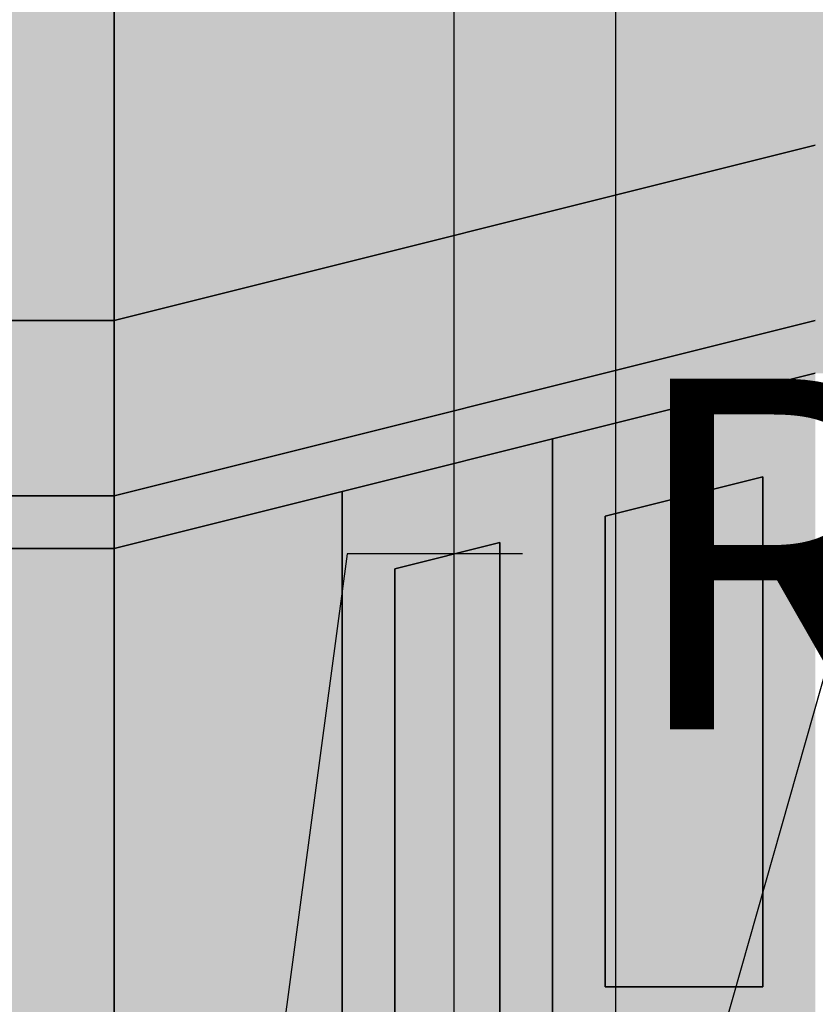
# Model space of a CAD drawing. Units: millimetres. Extents: x 130 to 1021, y 147 to 699.
# Tile 30 of 40: x 442 to 487, y 548 to 604. Entities that reach past the tile are written whole.
import ezdxf

# ---------------------------------------------------------------- set-up
doc = ezdxf.new("R2010")
doc.units = ezdxf.units.MM
doc.header["$MEASUREMENT"] = 0
for name, color, linetype, lineweight in [('A-ANNO-DIMS', 2, 'Continuous', 18), ('A-ELEV', 7, 'Continuous', 35), ('A-ELEV-PATT', 9, 'Continuous', 13)]:
    doc.layers.add(name, color=color, linetype=linetype, lineweight=lineweight)
doc.styles.get("Standard").update_dxf_attribs({"font": 'arial.ttf'})
doc.dimstyles.get("Standard").update_dxf_attribs({"dimtxt": 20, "dimasz": 10, "dimexe": 10, "dimexo": 10, "dimgap": 5, "dimtad": 0, "dimtih": 1, "dimtoh": 1, "dimdec": 0, "dimzin": 0, "dimdsep": 46, "dimtxsty": 'Standard', "dimcen": 5, "dimadec": 0, "dimazin": 0, "dimtfac": 1, "dimtdec": 0, "dimtofl": 0, "dimtmove": 0, "dimatfit": 3, "dimfxl": 1, "dimtolj": 1, "dimtzin": 0, "dimarcsym": 0})

# ---------------------------------------------------------------- blocks, each defined once
blk = doc.blocks.new('*D11')
at = {"layer": 'A-ANNO-DIMS', "color": 0, "lineweight": -2, "transparency": 16777216}
for p, q in [((737.374, 648.699), (737.374, 149.739)), ((299.374, 566.947), (299.374, 149.739)), ((309.374, 159.739), (490.857, 159.739)), ((727.374, 159.739), (545.891, 159.739))]:
    blk.add_line(p, q, dxfattribs=at)
at = {"layer": 'A-ANNO-DIMS', "color": 0, "transparency": 16777216}
for points in [[(309.374, 161.406), (309.374, 158.073), (299.374, 159.739)], [(727.374, 161.406), (727.374, 158.073), (737.374, 159.739)]]:
    blk.add_solid(points, dxfattribs=at)
at = {"layer": 'Defpoints', "color": 0, "transparency": 16777216}
for p in [(737.374, 658.699), (299.374, 576.947), (737.374, 159.739)]:
    blk.add_point(p, dxfattribs=at)
at = {"layer": 'A-ANNO-DIMS', "color": 0, "transparency": 16777216, "insert": (518.374, 159.739), "char_height": 20, "attachment_point": 5}
blk.add_mtext('\\A1;438', dxfattribs=at)
blk = doc.blocks.new('*D12')
at = {"layer": 'A-ANNO-DIMS', "color": 0, "lineweight": -2, "transparency": 16777216}
for p, q in [((477.374, 661.947), (265.074, 661.947)), ((275.074, 651.947), (275.074, 438.205)), ((275.074, 194.039), (275.074, 407.782)), ((357.163, 184.039), (265.074, 184.039))]:
    blk.add_line(p, q, dxfattribs=at)
at = {"layer": 'A-ANNO-DIMS', "color": 0, "transparency": 16777216}
for points in [[(273.407, 651.947), (276.74, 651.947), (275.074, 661.947)], [(273.407, 194.039), (276.74, 194.039), (275.074, 184.039)]]:
    blk.add_solid(points, dxfattribs=at)
at = {"layer": 'Defpoints', "color": 0, "transparency": 16777216}
for p in [(275.074, 661.947), (487.374, 661.947), (367.163, 184.039)]:
    blk.add_point(p, dxfattribs=at)
at = {"layer": 'A-ANNO-DIMS', "color": 0, "transparency": 16777216, "insert": (275.074, 422.993), "char_height": 20, "attachment_point": 5}
blk.add_mtext('\\A1;477.9', dxfattribs=at)
blk = doc.blocks.new('*D16')
at = {"layer": 'A-ANNO-DIMS', "color": 0, "lineweight": -2, "transparency": 16777216}
for p, q in [((357.941, 411.947), (357.941, 696.247)), ((363.922, 579.884), (363.922, 696.247)), ((347.941, 686.247), (337.941, 686.247)), ((373.922, 686.247), (383.922, 686.247))]:
    blk.add_line(p, q, dxfattribs=at)
at = {"layer": 'A-ANNO-DIMS', "color": 0, "transparency": 16777216}
for points in [[(347.941, 687.914), (347.941, 684.581), (357.941, 686.247)], [(373.922, 687.914), (373.922, 684.581), (363.922, 686.247)]]:
    blk.add_solid(points, dxfattribs=at)
at = {"layer": 'Defpoints', "color": 0, "transparency": 16777216}
for p in [(363.922, 686.247), (363.922, 569.884), (357.941, 401.947)]:
    blk.add_point(p, dxfattribs=at)
at = {"layer": 'A-ANNO-DIMS', "color": 0, "transparency": 16777216, "insert": (420.737, 686.247), "char_height": 20, "attachment_point": 5}
blk.add_mtext('\\A1;5.981', dxfattribs=at)
blk = doc.blocks.new('*D17')
at = {"layer": 'A-ANNO-DIMS', "color": 0, "lineweight": -2, "transparency": 16777216}
for p, q in [((363.922, 579.884), (363.922, 696.247)), ((375.85, 490.216), (375.85, 696.247)), ((353.922, 686.247), (343.922, 686.247)), ((385.85, 686.247), (395.85, 686.247))]:
    blk.add_line(p, q, dxfattribs=at)
at = {"layer": 'A-ANNO-DIMS', "color": 0, "transparency": 16777216}
for points in [[(353.922, 687.914), (353.922, 684.581), (363.922, 686.247)], [(385.85, 687.914), (385.85, 684.581), (375.85, 686.247)]]:
    blk.add_solid(points, dxfattribs=at)
at = {"layer": 'Defpoints', "color": 0, "transparency": 16777216}
for p in [(375.85, 686.247), (363.922, 569.884), (375.85, 480.216)]:
    blk.add_point(p, dxfattribs=at)
at = {"layer": 'A-ANNO-DIMS', "color": 0, "transparency": 16777216, "insert": (441.444, 686.247), "char_height": 20, "attachment_point": 5}
blk.add_mtext('\\A1;11.928', dxfattribs=at)
blk = doc.blocks.new('*D18')
at = {"layer": 'A-ANNO-DIMS', "color": 0, "lineweight": -2, "transparency": 16777216}
for p, q in [((375.85, 490.216), (375.85, 696.247)), ((382.374, 388.947), (382.374, 696.247)), ((365.85, 686.247), (355.85, 686.247)), ((392.374, 686.247), (402.374, 686.247))]:
    blk.add_line(p, q, dxfattribs=at)
at = {"layer": 'A-ANNO-DIMS', "color": 0, "transparency": 16777216}
for points in [[(365.85, 687.914), (365.85, 684.581), (375.85, 686.247)], [(392.374, 687.914), (392.374, 684.581), (382.374, 686.247)]]:
    blk.add_solid(points, dxfattribs=at)
at = {"layer": 'Defpoints', "color": 0, "transparency": 16777216}
for p in [(382.374, 686.247), (375.85, 480.216), (382.374, 378.947)]:
    blk.add_point(p, dxfattribs=at)
at = {"layer": 'A-ANNO-DIMS', "color": 0, "transparency": 16777216, "insert": (441.132, 686.247), "char_height": 20, "attachment_point": 5}
blk.add_mtext('\\A1;6.524', dxfattribs=at)
blk = doc.blocks.new('*D19')
at = {"layer": 'A-ANNO-DIMS', "color": 0, "lineweight": -2, "transparency": 16777216}
for p, q in [((382.374, 388.947), (382.374, 696.247)), ((414.652, 510.881), (414.652, 696.247)), ((392.374, 686.247), (404.652, 686.247)), ((414.652, 686.247), (424.652, 686.247))]:
    blk.add_line(p, q, dxfattribs=at)
at = {"layer": 'A-ANNO-DIMS', "color": 0, "transparency": 16777216}
for points in [[(392.374, 687.914), (392.374, 684.581), (382.374, 686.247)], [(404.652, 687.914), (404.652, 684.581), (414.652, 686.247)]]:
    blk.add_solid(points, dxfattribs=at)
at = {"layer": 'Defpoints', "color": 0, "transparency": 16777216}
for p in [(414.652, 686.247), (414.652, 500.881), (382.374, 378.947)]:
    blk.add_point(p, dxfattribs=at)
at = {"layer": 'A-ANNO-DIMS', "color": 0, "transparency": 16777216, "insert": (463.411, 686.247), "char_height": 20, "attachment_point": 5}
blk.add_mtext('\\A1;32.28', dxfattribs=at)
blk = doc.blocks.new('*D20')
at = {"layer": 'A-ANNO-DIMS', "color": 0, "lineweight": -2, "transparency": 16777216}
for p, q in [((414.652, 510.881), (414.652, 696.247)), ((432.374, 388.947), (432.374, 696.247)), ((404.652, 686.247), (394.652, 686.247)), ((442.374, 686.247), (452.374, 686.247))]:
    blk.add_line(p, q, dxfattribs=at)
at = {"layer": 'A-ANNO-DIMS', "color": 0, "transparency": 16777216}
for points in [[(404.652, 687.914), (404.652, 684.581), (414.652, 686.247)], [(442.374, 687.914), (442.374, 684.581), (432.374, 686.247)]]:
    blk.add_solid(points, dxfattribs=at)
at = {"layer": 'Defpoints', "color": 0, "transparency": 16777216}
for p in [(432.374, 686.247), (414.652, 500.881), (432.374, 378.947)]:
    blk.add_point(p, dxfattribs=at)
at = {"layer": 'A-ANNO-DIMS', "color": 0, "transparency": 16777216, "insert": (490.075, 686.247), "char_height": 20, "attachment_point": 5}
blk.add_mtext('\\A1;17.72', dxfattribs=at)
blk = doc.blocks.new('*D21')
at = {"layer": 'A-ANNO-DIMS', "color": 0, "lineweight": -2, "transparency": 16777216}
for p, q in [((432.374, 388.947), (432.374, 696.247)), ((447.374, 656.947), (447.374, 696.247)), ((422.374, 686.247), (412.374, 686.247)), ((457.374, 686.247), (467.374, 686.247))]:
    blk.add_line(p, q, dxfattribs=at)
at = {"layer": 'A-ANNO-DIMS', "color": 0, "transparency": 16777216}
for points in [[(422.374, 687.914), (422.374, 684.581), (432.374, 686.247)], [(457.374, 687.914), (457.374, 684.581), (447.374, 686.247)]]:
    blk.add_solid(points, dxfattribs=at)
at = {"layer": 'Defpoints', "color": 0, "transparency": 16777216}
for p in [(447.374, 686.247), (447.374, 646.947), (432.374, 378.947)]:
    blk.add_point(p, dxfattribs=at)
at = {"layer": 'A-ANNO-DIMS', "color": 0, "transparency": 16777216, "insert": (485.832, 686.247), "char_height": 20, "attachment_point": 5}
blk.add_mtext('\\A1;15', dxfattribs=at)
blk = doc.blocks.new('*D22')
at = {"layer": 'A-ANNO-DIMS', "color": 0, "lineweight": -2, "transparency": 16777216}
for p, q in [((447.374, 656.947), (447.374, 696.247)), ((466.767, 403.947), (466.767, 696.247)), ((437.374, 686.247), (427.374, 686.247)), ((476.767, 686.247), (486.767, 686.247))]:
    blk.add_line(p, q, dxfattribs=at)
at = {"layer": 'A-ANNO-DIMS', "color": 0, "transparency": 16777216}
for points in [[(437.374, 687.914), (437.374, 684.581), (447.374, 686.247)], [(476.767, 687.914), (476.767, 684.581), (466.767, 686.247)]]:
    blk.add_solid(points, dxfattribs=at)
at = {"layer": 'Defpoints', "color": 0, "transparency": 16777216}
for p in [(466.767, 686.247), (447.374, 646.947), (466.767, 393.947)]:
    blk.add_point(p, dxfattribs=at)
at = {"layer": 'A-ANNO-DIMS', "color": 0, "transparency": 16777216, "insert": (532.34, 686.247), "char_height": 20, "attachment_point": 5}
blk.add_mtext('\\A1;19.393', dxfattribs=at)
blk = doc.blocks.new('*D23')
at = {"layer": 'A-ANNO-DIMS', "color": 0, "lineweight": -2, "transparency": 16777216}
for p, q in [((466.767, 403.947), (466.767, 696.247)), ((475.988, 209.039), (475.988, 696.247)), ((456.767, 686.247), (446.767, 686.247)), ((485.988, 686.247), (495.988, 686.247))]:
    blk.add_line(p, q, dxfattribs=at)
at = {"layer": 'A-ANNO-DIMS', "color": 0, "transparency": 16777216}
for points in [[(456.767, 687.914), (456.767, 684.581), (466.767, 686.247)], [(485.988, 687.914), (485.988, 684.581), (475.988, 686.247)]]:
    blk.add_solid(points, dxfattribs=at)
at = {"layer": 'Defpoints', "color": 0, "transparency": 16777216}
for p in [(475.988, 686.247), (466.767, 393.947), (475.988, 199.039)]:
    blk.add_point(p, dxfattribs=at)
at = {"layer": 'A-ANNO-DIMS', "color": 0, "transparency": 16777216, "insert": (534.631, 686.247), "char_height": 20, "attachment_point": 5}
blk.add_mtext('\\A1;9.222', dxfattribs=at)
blk = doc.blocks.new('*D24')
at = {"layer": 'A-ANNO-DIMS', "color": 0, "lineweight": -2, "transparency": 16777216}
for p, q in [((475.988, 209.039), (475.988, 696.247)), ((487.374, 671.947), (487.374, 696.247)), ((465.988, 686.247), (455.988, 686.247)), ((497.374, 686.247), (507.374, 686.247))]:
    blk.add_line(p, q, dxfattribs=at)
at = {"layer": 'A-ANNO-DIMS', "color": 0, "transparency": 16777216}
for points in [[(465.988, 687.914), (465.988, 684.581), (475.988, 686.247)], [(497.374, 687.914), (497.374, 684.581), (487.374, 686.247)]]:
    blk.add_solid(points, dxfattribs=at)
at = {"layer": 'Defpoints', "color": 0, "transparency": 16777216}
for p in [(487.374, 686.247), (487.374, 661.947), (475.988, 199.039)]:
    blk.add_point(p, dxfattribs=at)
at = {"layer": 'A-ANNO-DIMS', "color": 0, "transparency": 16777216, "insert": (553.022, 686.247), "char_height": 20, "attachment_point": 5}
blk.add_mtext('\\A1;11.385', dxfattribs=at)
blk = doc.blocks.new('*D25')
at = {"layer": 'A-ANNO-DIMS', "color": 0, "lineweight": -2, "transparency": 16777216}
for p, q in [((487.374, 671.947), (487.374, 696.247)), ((494.102, 506.908), (494.102, 696.247)), ((477.374, 686.247), (467.374, 686.247)), ((504.102, 686.247), (514.102, 686.247))]:
    blk.add_line(p, q, dxfattribs=at)
at = {"layer": 'A-ANNO-DIMS', "color": 0, "transparency": 16777216}
for points in [[(477.374, 687.914), (477.374, 684.581), (487.374, 686.247)], [(504.102, 687.914), (504.102, 684.581), (494.102, 686.247)]]:
    blk.add_solid(points, dxfattribs=at)
at = {"layer": 'Defpoints', "color": 0, "transparency": 16777216}
for p in [(494.102, 686.247), (487.374, 661.947), (494.102, 496.908)]:
    blk.add_point(p, dxfattribs=at)
at = {"layer": 'A-ANNO-DIMS', "color": 0, "transparency": 16777216, "insert": (552.922, 686.247), "char_height": 20, "attachment_point": 5}
blk.add_mtext('\\A1;6.728', dxfattribs=at)
blk = doc.blocks.new('*D26')
at = {"layer": 'A-ANNO-DIMS', "color": 0, "lineweight": -2, "transparency": 16777216}
for p, q in [((494.102, 506.908), (494.102, 696.247)), ((502.374, 593.947), (502.374, 696.247)), ((484.102, 686.247), (474.102, 686.247)), ((512.374, 686.247), (522.374, 686.247))]:
    blk.add_line(p, q, dxfattribs=at)
at = {"layer": 'A-ANNO-DIMS', "color": 0, "transparency": 16777216}
for points in [[(484.102, 687.914), (484.102, 684.581), (494.102, 686.247)], [(512.374, 687.914), (512.374, 684.581), (502.374, 686.247)]]:
    blk.add_solid(points, dxfattribs=at)
at = {"layer": 'Defpoints', "color": 0, "transparency": 16777216}
for p in [(502.374, 686.247), (502.374, 583.947), (494.102, 496.908)]:
    blk.add_point(p, dxfattribs=at)
at = {"layer": 'A-ANNO-DIMS', "color": 0, "transparency": 16777216, "insert": (561.03, 686.247), "char_height": 20, "attachment_point": 5}
blk.add_mtext('\\A1;8.272', dxfattribs=at)
blk = doc.blocks.new('*D69')
at = {"layer": 'A-ANNO-DIMS', "color": 0, "lineweight": -2, "transparency": 16777216}
for p, q in [((507.746, 572.261), (483.091, 501.813)), ((517.746, 572.261), (507.746, 572.261)), ((433.191, 354.23), (433.191, 364.23)), ((428.191, 359.23), (438.191, 359.23))]:
    blk.add_line(p, q, dxfattribs=at)
at = {"layer": 'A-ANNO-DIMS', "color": 0, "transparency": 16777216}
blk.add_solid([(481.518, 502.363), (484.664, 501.262), (479.788, 492.374)], dxfattribs=at)
at = {"layer": 'Defpoints', "color": 0, "transparency": 16777216}
for p in [(479.788, 492.374), (433.191, 359.23)]:
    blk.add_point(p, dxfattribs=at)
at = {"layer": 'A-ANNO-DIMS', "color": 0, "transparency": 16777216, "insert": (573.824, 572.261), "char_height": 20, "attachment_point": 5}
blk.add_mtext('\\A1;R141.06', dxfattribs=at)
blk = doc.blocks.new('*D71')
at = {"layer": 'A-ANNO-DIMS', "color": 0, "lineweight": -2, "transparency": 16777216}
for p, q in [((492.108, 581.609), (472.542, 512.666)), ((502.108, 581.609), (492.108, 581.609)), ((432.65, 367.109), (432.65, 377.109)), ((427.65, 372.109), (437.65, 372.109))]:
    blk.add_line(p, q, dxfattribs=at)
at = {"layer": 'A-ANNO-DIMS', "color": 0, "transparency": 16777216}
blk.add_solid([(470.938, 513.121), (474.145, 512.211), (469.812, 503.046)], dxfattribs=at)
at = {"layer": 'Defpoints', "color": 0, "transparency": 16777216}
for p in [(469.812, 503.046), (432.65, 372.109)]:
    blk.add_point(p, dxfattribs=at)
at = {"layer": 'A-ANNO-DIMS', "color": 0, "transparency": 16777216, "insert": (548.493, 581.609), "char_height": 20, "attachment_point": 5}
blk.add_mtext('\\A1;R136.1', dxfattribs=at)
blk = doc.blocks.new('*D72')
at = {"layer": 'A-ANNO-DIMS', "color": 0, "lineweight": -2, "transparency": 16777216}
for p, q in [((460.658, 573.64), (451.279, 503.49)), ((470.658, 573.64), (460.658, 573.64)), ((432.115, 355.142), (432.115, 365.142)), ((427.115, 360.142), (437.115, 360.142))]:
    blk.add_line(p, q, dxfattribs=at)
at = {"layer": 'A-ANNO-DIMS', "color": 0, "transparency": 16777216}
blk.add_solid([(449.628, 503.711), (452.931, 503.27), (449.954, 493.579)], dxfattribs=at)
at = {"layer": 'Defpoints', "color": 0, "transparency": 16777216}
for p in [(449.954, 493.579), (432.115, 360.142)]:
    blk.add_point(p, dxfattribs=at)
at = {"layer": 'A-ANNO-DIMS', "color": 0, "transparency": 16777216, "insert": (526.64, 573.64), "char_height": 20, "attachment_point": 5}
blk.add_mtext('\\A1;R134.62', dxfattribs=at)

msp = doc.modelspace()

# ---------------------------------------------------------------- hatches: boundary and pattern name
at = {"layer": 'A-ELEV-PATT'}
h = msp.add_hatch(color=256, dxfattribs=at)
h.dxf.hatch_style = 1
h.paths.add_polyline_path([(737.3738, 658.6988, 0.0135961), (632.4019, 661.9473), (607.3738, 661.9473), (487.3738, 661.9473), (487.3738, 649.9473), (607.3738, 649.9473), (632.3794, 649.9473, -0.0136841), (737.3738, 646.6784)])
h.paths.add_polyline_path([(732.3738, 643.9599, 0.0130529), (632.3738, 646.9473), (607.3738, 646.9473), (487.3738, 646.9473), (487.3738, 596.9473), (632.3738, 596.9473, -0.0130529), (732.3738, 593.9599)])
h.paths.add_polyline_path([(737.3738, 593.6732, 0.0137063), (632.3738, 596.9473), (487.3738, 596.9473), (487.3738, 586.9473), (632.355, 586.9473, -0.0137808), (737.3738, 583.6559)])
h.paths.add_polyline_path([(447.3738, 646.9473), (307.3738, 646.9473), (302.3738, 646.9473), (302.3738, 634.9473), (447.3738, 634.9473)])
h.paths.add_polyline_path([(447.3738, 631.9473), (307.3738, 631.9473), (307.3738, 586.9473), (447.3738, 586.9473)])
h.paths.add_polyline_path([(447.3738, 586.9473), (307.3738, 586.9473), (302.3738, 586.9473), (302.3738, 576.9473), (447.3738, 576.9473)])
h.paths.add_polyline_path([(447.3738, 573.9473), (367.3738, 573.9473), (367.3738, 539.9473), (447.3738, 539.9473)])
h.paths.add_polyline_path([(447.3738, 537.9473), (367.3738, 537.9473), (367.3738, 507.9473), (400.392, 507.4253, -0.001728), (401.3281, 507.6451, -0.5220025), (425.6117, 511.0391, -0.0391849), (447.3738, 510.4359), (447.3738, 510.7883)])
h.paths.add_polyline_path([(394.7238, 505.9473), (367.3738, 505.9473), (367.3738, 476.9473, -0.0146512), (375.8501, 480.2159), (376.1506, 499.2266, -0.0355419)])
h.paths.add_polyline_path([(632.3738, 583.9473), (552.3738, 583.9473), (552.3738, 550.9473), (632.3738, 550.9473)])
h.paths.add_polyline_path([(632.3738, 548.9473), (552.3738, 548.9473), (552.3738, 515.9473), (632.3738, 515.9473)])
h.paths.add_polyline_path([(632.3738, 513.9473), (552.3738, 513.9473), (552.3738, 476.9473), (632.3738, 476.9473)])
h.paths.add_polyline_path([(737.3738, 473.6903, 0.0136326), (632.3926, 476.9473), (552.3738, 476.9473), (487.3738, 476.9473), (487.3738, 466.9473), (632.3738, 466.9473, -0.0137063), (737.3738, 463.6732)])
h.paths.add_polyline_path([(732.3738, 460.9552, 0.0130741), (632.3681, 463.9473), (487.3738, 463.9473), (487.3738, 407.735, -0.0032286), (489.3544, 406.9473), (632.3926, 406.9473, -0.0129826), (732.3738, 403.9755)])
h.paths.add_polyline_path([(487.3738, 463.9473, 0.20133), (367.3738, 463.9473), (367.3738, 407.735, -0.1882031), (487.3738, 407.735)])
h.paths.add_polyline_path([(367.3738, 476.9473), (367.3738, 466.9473, -0.2013309), (487.3738, 466.9473), (487.3738, 476.9473, 0.20133)])
h.paths.add_polyline_path([(367.3738, 463.9473), (307.3738, 463.9473), (307.3738, 401.9473), (357.9413, 401.9473), (367.3738, 407.735)])
h.paths.add_polyline_path([(367.3738, 476.9473), (302.3738, 476.9473), (302.3738, 466.9473), (367.3738, 466.9473)])
h.paths.add_polyline_path([(632.8184, 366.9453), (552.3738, 366.9453), (552.3738, 393.9473), (632.8184, 393.9473)])
h.paths.add_polyline_path([(632.8184, 357.2114), (632.8184, 363.9453), (552.3738, 363.9453), (552.3738, 357.2114), (552.3738, 336.9453), (632.8184, 336.9453)])
h.paths.add_polyline_path([(632.8184, 333.9453), (552.3738, 333.9453), (552.3738, 306.9453), (632.8184, 306.9453)])
h.paths.add_polyline_path([(632.8184, 303.9453), (552.3738, 303.9453), (552.3738, 273.9473), (632.355, 273.9473, 0.0000608), (632.8184, 273.9491)])
h.paths.add_polyline_path([(737.3738, 403.6903, 0.0136326), (632.3926, 406.9473), (489.3544, 406.9473, 0.1915481), (367.3738, 407.735), (367.3738, 396.9473, -0.2013309), (487.3738, 396.9473), (632.3738, 396.9473, -0.0137063), (737.3738, 393.6732)])
h.paths.add_polyline_path([(357.9413, 401.9473), (307.3738, 401.9473), (307.3738, 391.9473), (357.9413, 391.9473)])
h.paths.add_polyline_path([(357.9413, 357.2114), (357.9413, 388.9473), (307.3738, 388.9473), (307.3738, 357.2114), (307.3738, 273.9473), (357.9413, 273.9473)])
h.paths.add_polyline_path([(732.3738, 263.93, -0.0130317), (632.3794, 260.9473), (466.7667, 260.9473), (466.7667, 240.9473), (469.8406, 236.978), (469.8406, 221.978), (472.9145, 218.0087), (472.9145, 213.9473), (607.3738, 213.9473), (732.3738, 213.9473)])
h.paths.add_polyline_path([(732.3738, 290.889), (722.479, 290.889), (722.479, 301.889), (732.3738, 301.889), (732.3738, 305.889), (722.479, 305.889), (722.479, 316.889), (732.3738, 316.889), (732.3738, 320.889), (722.479, 320.889), (722.479, 331.889), (732.3738, 331.889), (732.3738, 335.889), (722.479, 335.889), (722.479, 346.889), (732.3738, 346.889), (732.3738, 350.889), (722.479, 350.889), (722.479, 361.889), (732.3738, 361.889), (732.3738, 365.889), (722.479, 365.889), (722.479, 376.889), (732.3738, 376.889), (732.3738, 380.889), (722.479, 380.889), (722.479, 391.4848, 0.0005233), (718.479, 391.6843), (718.479, 380.889), (707.479, 380.889), (707.479, 392.1896, 0.0005231), (703.479, 392.3576), (703.479, 380.889), (692.479, 380.889), (692.479, 392.7765, 0.0005229), (688.479, 392.9131), (688.479, 380.889), (677.479, 380.889), (677.479, 393.2456, 0.0005228), (673.479, 393.3508), (673.479, 380.889), (662.479, 380.889), (662.479, 393.597, 0.0005227), (658.479, 393.6709), (658.479, 380.889), (647.479, 380.889), (647.479, 393.8308, 0.0005226), (643.479, 393.8732), (643.479, 380.889), (632.8184, 380.889), (632.8184, 376.889), (643.479, 376.889), (643.479, 365.889), (632.8184, 365.889), (632.8184, 361.889), (643.479, 361.889), (643.479, 350.889), (632.8184, 350.889), (632.8184, 346.889), (643.479, 346.889), (643.479, 335.889), (632.8184, 335.889), (632.8184, 331.889), (643.479, 331.889), (643.479, 320.889), (632.8184, 320.889), (632.8184, 316.889), (643.479, 316.889), (643.479, 305.889), (632.8184, 305.889), (632.8184, 301.889), (643.479, 301.889), (643.479, 290.889), (632.8184, 290.889), (632.8184, 286.889), (643.479, 286.889), (643.479, 274.0217, 0.0005246), (647.479, 274.0643), (647.479, 286.889), (658.479, 286.889), (658.479, 274.2248, 0.0005246), (662.479, 274.2989), (662.479, 286.889), (673.479, 286.889), (673.479, 274.546, 0.0005247), (677.479, 274.6516), (677.479, 286.889), (688.479, 286.889), (688.479, 274.9853, 0.0005248), (692.479, 275.1224), (692.479, 286.889), (703.479, 286.889), (703.479, 275.5429, 0.000525), (707.479, 275.7115), (707.479, 286.889), (718.479, 286.889), (718.479, 276.2187, 0.0005252), (722.479, 276.4189), (722.479, 286.889), (732.3738, 286.889)])
h.paths.add_polyline_path([(718.479, 290.889), (707.479, 290.889), (707.479, 301.889), (718.479, 301.889)], flags=16)
h.paths.add_polyline_path([(703.479, 290.889), (692.479, 290.889), (692.479, 301.889), (703.479, 301.889)], flags=16)
h.paths.add_polyline_path([(718.479, 305.889), (707.479, 305.889), (707.479, 316.889), (718.479, 316.889)], flags=16)
h.paths.add_polyline_path([(703.479, 305.889), (692.479, 305.889), (692.479, 316.889), (703.479, 316.889)], flags=16)
h.paths.add_polyline_path([(688.479, 290.889), (677.479, 290.889), (677.479, 301.889), (688.479, 301.889)], flags=16)
h.paths.add_polyline_path([(718.479, 320.889), (707.479, 320.889), (707.479, 331.889), (718.479, 331.889)], flags=16)
h.paths.add_polyline_path([(688.479, 305.889), (677.479, 305.889), (677.479, 316.889), (688.479, 316.889)], flags=16)
h.paths.add_polyline_path([(703.479, 320.889), (692.479, 320.889), (692.479, 331.889), (703.479, 331.889)], flags=16)
h.paths.add_polyline_path([(688.479, 320.889), (677.479, 320.889), (677.479, 331.889), (688.479, 331.889)], flags=16)
h.paths.add_polyline_path([(673.479, 290.889), (662.479, 290.889), (662.479, 301.889), (673.479, 301.889)], flags=16)
h.paths.add_polyline_path([(718.479, 335.889), (707.479, 335.889), (707.479, 346.889), (718.479, 346.889)], flags=16)
h.paths.add_polyline_path([(673.479, 305.889), (662.479, 305.889), (662.479, 316.889), (673.479, 316.889)], flags=16)
h.paths.add_polyline_path([(703.479, 335.889), (692.479, 335.889), (692.479, 346.889), (703.479, 346.889)], flags=16)
h.paths.add_polyline_path([(673.479, 320.889), (662.479, 320.889), (662.479, 331.889), (673.479, 331.889)], flags=16)
h.paths.add_polyline_path([(688.479, 335.889), (677.479, 335.889), (677.479, 346.889), (688.479, 346.889)], flags=16)
h.paths.add_polyline_path([(658.479, 290.889), (647.479, 290.889), (647.479, 301.889), (658.479, 301.889)], flags=16)
h.paths.add_polyline_path([(718.479, 350.889), (707.479, 350.889), (707.479, 361.889), (718.479, 361.889)], flags=16)
h.paths.add_polyline_path([(658.479, 305.889), (647.479, 305.889), (647.479, 316.889), (658.479, 316.889)], flags=16)
h.paths.add_polyline_path([(703.479, 350.889), (692.479, 350.889), (692.479, 361.889), (703.479, 361.889)], flags=16)
h.paths.add_polyline_path([(673.479, 335.889), (662.479, 335.889), (662.479, 346.889), (673.479, 346.889)], flags=16)
h.paths.add_polyline_path([(658.479, 320.889), (647.479, 320.889), (647.479, 331.889), (658.479, 331.889)], flags=16)
h.paths.add_polyline_path([(688.479, 350.889), (677.479, 350.889), (677.479, 361.889), (688.479, 361.889)], flags=16)
h.paths.add_polyline_path([(718.479, 365.889), (707.479, 365.889), (707.479, 376.889), (718.479, 376.889)], flags=16)
h.paths.add_polyline_path([(658.479, 335.889), (647.479, 335.889), (647.479, 346.889), (658.479, 346.889)], flags=16)
h.paths.add_polyline_path([(673.479, 350.889), (662.479, 350.889), (662.479, 361.889), (673.479, 361.889)], flags=16)
h.paths.add_polyline_path([(703.479, 365.889), (692.479, 365.889), (692.479, 376.889), (703.479, 376.889)], flags=16)
h.paths.add_polyline_path([(688.479, 365.889), (677.479, 365.889), (677.479, 376.889), (688.479, 376.889)], flags=16)
h.paths.add_polyline_path([(658.479, 350.889), (647.479, 350.889), (647.479, 361.889), (658.479, 361.889)], flags=16)
h.paths.add_polyline_path([(673.479, 365.889), (662.479, 365.889), (662.479, 376.889), (673.479, 376.889)], flags=16)
h.paths.add_polyline_path([(658.479, 365.889), (647.479, 365.889), (647.479, 376.889), (658.479, 376.889)], flags=16)
h.paths.add_polyline_path([(732.3738, 503.9786), (722.3392, 503.9786), (722.3392, 514.9786), (732.3738, 514.9786), (732.3738, 518.9786), (722.3392, 518.9786), (722.3392, 529.9786), (732.3738, 529.9786), (732.3738, 533.9786), (722.3392, 533.9786), (722.3392, 544.9786), (732.3738, 544.9786), (732.3738, 546.9473), (732.3738, 548.9786), (722.3392, 548.9786), (722.3392, 559.9786), (732.3738, 559.9786), (732.3738, 563.9786), (722.3392, 563.9786), (722.3392, 574.9786), (732.3738, 574.9786), (732.3738, 578.9786), (722.3392, 578.9786), (722.3392, 581.4789, 0.000526), (718.3392, 581.6791), (718.3392, 578.9786), (707.3392, 578.9786), (707.3392, 582.1863, 0.0005258), (703.3392, 582.355), (703.3392, 578.9786), (692.3392, 578.9786), (692.3392, 582.7752, 0.0005257), (688.3392, 582.9123), (688.3392, 578.9786), (677.3392, 578.9786), (677.3392, 583.2457, 0.0005255), (673.3392, 583.3512), (673.3392, 578.9786), (662.3392, 578.9786), (662.3392, 583.5978, 0.0005254), (658.3392, 583.6718), (658.3392, 578.9786), (647.3392, 578.9786), (647.3392, 583.8317, 0.0005254), (643.3392, 583.8741), (643.3392, 578.9786), (632.3738, 578.9786), (632.3738, 574.9786), (643.3392, 574.9786), (643.3392, 563.9786), (632.3738, 563.9786), (632.3738, 559.9786), (643.3392, 559.9786), (643.3392, 548.9786), (632.3738, 548.9786), (632.3738, 544.9786), (643.3392, 544.9786), (643.3392, 533.9786), (632.3738, 533.9786), (632.3738, 529.9786), (643.3392, 529.9786), (643.3392, 518.9786), (632.3738, 518.9786), (632.3738, 515.9473), (632.3738, 514.9786), (643.3392, 514.9786), (643.3392, 503.9786), (632.3738, 503.9786), (632.3738, 499.9786), (643.3392, 499.9786), (643.3392, 488.9786), (632.3738, 488.9786), (632.3738, 484.9786), (643.3392, 484.9786), (643.3392, 476.8751, -0.0005191), (647.3392, 476.8332), (647.3392, 484.9786), (658.3392, 484.9786), (658.3392, 476.6752, -0.0005192), (662.3392, 476.6022), (662.3392, 484.9786), (673.3392, 484.9786), (673.3392, 476.3585, -0.0005193), (677.3392, 476.2543), (677.3392, 484.9786), (688.3392, 484.9786), (688.3392, 475.9248, -0.0005194), (692.3392, 475.7894), (692.3392, 484.9786), (703.3392, 484.9786), (703.3392, 475.3741, -0.0005195), (707.3392, 475.2075), (707.3392, 484.9786), (718.3392, 484.9786), (718.3392, 474.7064, -0.0005197), (722.3392, 474.5086), (722.3392, 484.9786), (732.3738, 484.9786), (732.3738, 488.9786), (722.3392, 488.9786), (722.3392, 499.9786), (732.3738, 499.9786)])
h.paths.add_polyline_path([(718.3392, 503.9786), (707.3392, 503.9786), (707.3392, 514.9786), (718.3392, 514.9786)], flags=16)
h.paths.add_polyline_path([(718.3392, 499.9786), (718.3392, 488.9786), (707.3392, 488.9786), (707.3392, 499.9786)], flags=16)
h.paths.add_polyline_path([(718.3392, 518.9786), (707.3392, 518.9786), (707.3392, 529.9786), (718.3392, 529.9786)], flags=16)
h.paths.add_polyline_path([(703.3392, 503.9786), (692.3392, 503.9786), (692.3392, 514.9786), (703.3392, 514.9786)], flags=16)
h.paths.add_polyline_path([(703.3392, 499.9786), (703.3392, 488.9786), (692.3392, 488.9786), (692.3392, 499.9786)], flags=16)
h.paths.add_polyline_path([(703.3392, 518.9786), (692.3392, 518.9786), (692.3392, 529.9786), (703.3392, 529.9786)], flags=16)
h.paths.add_polyline_path([(718.3392, 533.9786), (707.3392, 533.9786), (707.3392, 544.9786), (718.3392, 544.9786)], flags=16)
h.paths.add_polyline_path([(688.3392, 503.9786), (677.3392, 503.9786), (677.3392, 514.9786), (688.3392, 514.9786)], flags=16)
h.paths.add_polyline_path([(688.3392, 499.9786), (688.3392, 488.9786), (677.3392, 488.9786), (677.3392, 499.9786)], flags=16)
h.paths.add_polyline_path([(703.3392, 533.9786), (692.3392, 533.9786), (692.3392, 544.9786), (703.3392, 544.9786)], flags=16)
h.paths.add_polyline_path([(688.3392, 518.9786), (677.3392, 518.9786), (677.3392, 529.9786), (688.3392, 529.9786)], flags=16)
h.paths.add_polyline_path([(688.3392, 533.9786), (677.3392, 533.9786), (677.3392, 544.9786), (688.3392, 544.9786)], flags=16)
h.paths.add_polyline_path([(718.3392, 548.9786), (707.3392, 548.9786), (707.3392, 559.9786), (718.3392, 559.9786)], flags=16)
h.paths.add_polyline_path([(673.3392, 503.9786), (662.3392, 503.9786), (662.3392, 514.9786), (673.3392, 514.9786)], flags=16)
h.paths.add_polyline_path([(673.3392, 499.9786), (673.3392, 488.9786), (662.3392, 488.9786), (662.3392, 499.9786)], flags=16)
h.paths.add_polyline_path([(703.3392, 548.9786), (692.3392, 548.9786), (692.3392, 559.9786), (703.3392, 559.9786)], flags=16)
h.paths.add_polyline_path([(673.3392, 518.9786), (662.3392, 518.9786), (662.3392, 529.9786), (673.3392, 529.9786)], flags=16)
h.paths.add_polyline_path([(688.3392, 548.9786), (677.3392, 548.9786), (677.3392, 559.9786), (688.3392, 559.9786)], flags=16)
h.paths.add_polyline_path([(673.3392, 533.9786), (662.3392, 533.9786), (662.3392, 544.9786), (673.3392, 544.9786)], flags=16)
h.paths.add_polyline_path([(718.3392, 563.9786), (707.3392, 563.9786), (707.3392, 574.9786), (718.3392, 574.9786)], flags=16)
h.paths.add_polyline_path([(658.3392, 503.9786), (647.3392, 503.9786), (647.3392, 514.9786), (658.3392, 514.9786)], flags=16)
h.paths.add_polyline_path([(658.3392, 499.9786), (658.3392, 488.9786), (647.3392, 488.9786), (647.3392, 499.9786)], flags=16)
h.paths.add_polyline_path([(703.3392, 563.9786), (692.3392, 563.9786), (692.3392, 574.9786), (703.3392, 574.9786)], flags=16)
h.paths.add_polyline_path([(658.3392, 518.9786), (647.3392, 518.9786), (647.3392, 529.9786), (658.3392, 529.9786)], flags=16)
h.paths.add_polyline_path([(673.3392, 548.9786), (662.3392, 548.9786), (662.3392, 559.9786), (673.3392, 559.9786)], flags=16)
h.paths.add_polyline_path([(688.3392, 563.9786), (677.3392, 563.9786), (677.3392, 574.9786), (688.3392, 574.9786)], flags=16)
h.paths.add_polyline_path([(658.3392, 533.9786), (647.3392, 533.9786), (647.3392, 544.9786), (658.3392, 544.9786)], flags=16)
h.paths.add_polyline_path([(673.3392, 563.9786), (662.3392, 563.9786), (662.3392, 574.9786), (673.3392, 574.9786)], flags=16)
h.paths.add_polyline_path([(658.3392, 548.9786), (647.3392, 548.9786), (647.3392, 559.9786), (658.3392, 559.9786)], flags=16)
h.paths.add_polyline_path([(658.3392, 563.9786), (647.3392, 563.9786), (647.3392, 574.9786), (658.3392, 574.9786)], flags=16)
h = msp.add_hatch(color=256, dxfattribs=at)
h.dxf.hatch_style = 1
h.paths.add_polyline_path([(487.3738, 649.9473), (487.3738, 661.9473), (447.3738, 646.9473), (447.3738, 634.9473)])
h.paths.add_polyline_path([(487.3738, 646.9473), (447.3738, 631.9473), (447.3738, 586.9473), (487.3738, 596.9473)])
h.paths.add_polyline_path([(487.3738, 596.9473), (447.3738, 586.9473), (447.3738, 576.9473), (487.3738, 586.9473)])
h.paths.add_polyline_path([(460.3738, 577.1973), (447.3738, 573.9473), (447.3738, 510.7883), (447.3738, 510.4359, -0.0236536), (460.3738, 508.4268), (460.3738, 509.3636)])
h.paths.add_polyline_path([(472.3738, 580.1973), (460.3738, 577.1973), (460.3738, 509.3636), (460.3738, 508.4268, -0.0055147), (463.3738, 507.7821), (463.3738, 508.8807), (463.3738, 572.7934), (469.3738, 574.2934), (469.3738, 507.7378), (469.3738, 506.2825, -0.0056075), (472.3738, 505.4251), (472.3738, 507.0765)])
h = msp.add_hatch(color=256, dxfattribs=at)
h.dxf.hatch_style = 1
h.paths.add_polyline_path([(447.3738, 576.9473), (302.3738, 576.9473), (302.3738, 573.9473), (447.3738, 573.9473)])
h.paths.add_polyline_path([(487.3738, 583.9473), (487.3738, 586.9473), (447.3738, 576.9473), (447.3738, 573.9473)])
h.paths.add_polyline_path([(632.355, 586.9473), (487.3738, 586.9473), (487.3738, 583.9473), (632.3738, 583.9473), (632.3738, 583.9472, -0.0138), (737.3738, 580.6507), (737.3738, 583.6559, 0.0137808)])
h.paths.add_polyline_path([(367.3738, 466.9473), (302.3738, 466.9473), (302.3738, 463.9473), (367.3738, 463.9473)])
h.paths.add_polyline_path([(487.3738, 463.9473), (487.3738, 466.9473, 0.2013309), (367.3738, 466.9473), (367.3738, 463.9473, -0.20133)])
h.paths.add_polyline_path([(632.3738, 466.9473), (487.3738, 466.9473), (487.3738, 463.9473), (632.3681, 463.9473, -0.0137285), (737.3738, 460.6681), (737.3738, 463.6732, 0.0137063)])
h.paths.add_polyline_path([(632.3738, 396.9473), (487.3738, 396.9473, 0.2013309), (367.3738, 396.9473), (367.3738, 393.9473, -0.2023717), (486.7667, 393.9473), (632.3681, 393.9473, -0.0137285), (737.3738, 390.6681), (737.3738, 393.6732, 0.0137063)])
h.paths.add_polyline_path([(357.9413, 391.9473), (307.3738, 391.9473), (307.3738, 388.9473), (357.9413, 388.9473)])
h.paths.add_polyline_path([(367.3738, 393.9473), (367.3738, 396.9473), (357.9413, 391.924), (357.9413, 388.9473), (358.058, 388.9473)])
h.paths.add_polyline_path([(737.3738, 264.2162), (737.3738, 267.2214, -0.0137063), (632.3738, 263.9473), (463.7667, 263.9473), (466.7667, 260.9473), (632.3794, 260.9473, 0.0136841)])
h.paths.add_polyline_path([(463.7667, 263.9473), (447.3738, 263.9473), (450.3738, 260.9473), (466.7667, 260.9473)])
h.paths.add_polyline_path([(447.3738, 263.9473), (432.3738, 263.9473), (432.3738, 260.9473), (450.3738, 260.9473)])
h.paths.add_polyline_path([(382.3738, 263.9473), (357.9413, 263.9473), (357.9413, 260.9473), (382.3738, 260.9473)])
h.paths.add_polyline_path([(357.9413, 263.9473), (307.3738, 263.9473), (307.3738, 260.9473), (357.9413, 260.9473)])
h = msp.add_hatch(color=256, dxfattribs=at)
h.paths.add_polyline_path([(327.3738, 569.884), (327.3738, 573.9473), (307.3738, 573.9473), (307.3738, 476.9473), (327.3738, 476.9473), (327.3738, 480.95)])
h.paths.add_polyline_path([(486.7667, 386.2639), (486.7667, 393.9473), (466.7667, 393.9473), (466.7667, 357.2114), (466.7667, 311.9335, 0.0342703), (486.7667, 308.4637)])
h.paths.add_polyline_path([(486.7667, 308.4637, -0.0342703), (466.7667, 311.9335), (466.7667, 273.9473), (486.7667, 273.9473)])
h.paths.add_polyline_path([(389.3738, 351.5473), (396.7693, 351.5473, -0.007027), (393.8774, 354.5473), (389.3738, 354.5473), (389.3738, 359.5775, -0.0190302), (382.3738, 368.424), (382.3738, 249.5473), (432.3738, 249.5473), (432.3738, 325.067, -0.0057673), (429.3738, 326.709), (429.3738, 257.5473), (426.3738, 257.5473), (426.3738, 328.4428, -0.0059254), (423.3738, 330.272), (423.3738, 315.7473), (389.3738, 315.7473), (389.3738, 332.1473), (420.4552, 332.1473, -0.008951), (416.0768, 335.1473), (389.3738, 335.1473)])
h.paths.add_polyline_path([(389.3738, 312.7473), (423.3738, 312.7473), (423.3738, 296.3473), (389.3738, 296.3473)], flags=16)
h.paths.add_polyline_path([(389.3738, 293.3473), (423.3738, 293.3473), (423.3738, 276.9473), (389.3738, 276.9473)], flags=16)
h.paths.add_polyline_path([(389.3738, 273.9473), (423.3738, 273.9473), (423.3738, 257.5473), (389.3738, 257.5473)], flags=16)
h.paths.add_polyline_path([(432.3738, 378.9473), (382.3738, 378.9473), (382.3738, 368.424, 0.0190302), (389.3738, 359.5775), (389.3738, 370.9473), (423.3738, 370.9473), (423.3738, 354.5473), (393.8774, 354.5473, 0.007027), (396.7693, 351.5473), (423.3738, 351.5473), (423.3738, 335.1473), (416.0768, 335.1473, 0.008951), (420.4552, 332.1473), (423.3738, 332.1473), (423.3738, 330.272, 0.0059254), (426.3738, 328.4428), (426.3738, 370.9473), (429.3738, 370.9473), (429.3738, 326.709, 0.0057673), (432.3738, 325.067)])
h.paths.add_polyline_path([(466.7667, 357.2114), (466.7667, 393.9473), (447.3738, 393.9473), (447.3738, 357.2114), (447.3738, 318.1243, 0.0063261), (450.8779, 316.785), (450.8779, 331.5915), (463.5608, 331.5915), (463.5608, 312.7571, 0.005582), (466.7667, 311.9335)])
h.paths.add_polyline_path([(450.8779, 334.5915), (450.8779, 360.0915), (463.5608, 360.0915), (463.5608, 334.5915)], flags=16)
h.paths.add_polyline_path([(450.8779, 363.0915), (450.8779, 388.6449), (463.5608, 388.6449), (463.5608, 363.0915)], flags=16)
h.paths.add_polyline_path([(466.7667, 311.9335, -0.005582), (463.5608, 312.7571), (463.5608, 306.0915), (450.8779, 306.0915), (450.8779, 316.785, -0.0063261), (447.3738, 318.1243), (447.3738, 273.9473), (466.7667, 273.9473)])
h.paths.add_polyline_path([(450.8779, 303.0915), (463.5608, 303.0915), (463.5608, 277.5915), (450.8779, 277.5915)], flags=16)
h.paths.add_polyline_path([(552.3738, 357.2114), (552.3738, 393.9473), (486.7667, 393.9473), (486.7667, 386.2639), (544.6354, 386.2639), (544.6354, 280.6619), (486.7667, 280.6619), (486.7667, 273.9473), (552.3738, 273.9473)])
h.paths.add_polyline_path([(487.3738, 583.9473), (472.3738, 580.1973), (472.3738, 507.0765), (472.3738, 505.4251, -0.0056452), (475.3738, 504.4942), (475.3738, 506.3543), (475.3738, 511.9473), (484.3738, 511.9473), (484.3738, 503.8134), (484.3738, 501.2439, -0.0058357), (487.3738, 500.0015)])
h.paths.add_polyline_path([(484.3738, 578.0434), (484.3738, 548.9473), (475.3738, 548.9473), (475.3738, 575.7934)], flags=16)
h.paths.add_polyline_path([(484.3738, 546.9473), (484.3738, 513.9473), (475.3738, 513.9473), (475.3738, 518.7148), (475.3738, 546.9473)], flags=16)
h = msp.add_hatch(color=256, dxfattribs=at)
h.set_gradient(color1=(221, 197, 207), color2=(128, 128, 128), name='INVCYLINDER')
h.paths.add_polyline_path([(475.3738, 548.9473), (484.3738, 548.9473), (484.3738, 578.0434), (475.3738, 575.7934)])
h.paths.add_polyline_path([(475.3738, 513.9473), (484.3738, 513.9473), (484.3738, 546.9473), (475.3738, 546.9473)])
h.paths.add_polyline_path([(475.3738, 511.9473), (475.3738, 506.3543), (475.3738, 504.4942, -0.017202), (484.3738, 501.2439), (484.3738, 503.8134), (484.3738, 511.9473)])
h.paths.add_polyline_path([(475.3738, 501.3382), (475.3738, 495.9324, -0.0166439), (484.3738, 492.8236), (484.3738, 498.0065, 0.0176328)])
h.paths.add_polyline_path([(475.3738, 493.8379), (475.3738, 487.6263, -0.0178833), (484.3738, 484.2088), (484.3738, 490.6796, 0.0169089)])
h.paths.add_polyline_path([(484.3738, 478.1696), (484.3738, 482.0358, 0.0181932), (475.3738, 485.5124), (475.3738, 481.4101, -0.0154272)])
msp.add_hatch(color=256, dxfattribs=at).paths.add_polyline_path([(469.3738, 574.2934), (463.3738, 572.7934), (463.3738, 508.8807), (463.3738, 507.7821, -0.011116), (469.3738, 506.2825), (469.3738, 507.7378)])

# ---------------------------------------------------------------- linework, layer by layer
at = {"layer": 'A-ELEV'}
for p, q in [((447.3738, 646.9473), (447.3738, 510.7883)), ((447.3738, 596.9473), (447.3738, 588.9473)), ((447.3738, 586.9473), (487.3738, 596.9473)), ((447.3738, 586.9473), (302.3738, 586.9473)), ((447.3738, 576.9473), (487.3738, 586.9473)), ((447.3738, 573.9473), (487.3738, 583.9473)), ((472.3738, 580.1973), (472.3738, 507.0765)), ((475.3738, 575.7934), (484.3738, 578.0434)), ((484.3738, 548.9473), (484.3738, 578.0434)), ((447.3738, 576.9473), (302.3738, 576.9473)), ((460.3738, 577.1973), (460.3738, 509.3636)), ((475.3738, 575.7934), (475.3738, 548.9473)), ((463.3738, 572.7934), (469.3738, 574.2934)), ((469.3738, 574.2934), (469.3738, 507.7378)), ((447.3738, 573.9473), (302.3738, 573.9473)), ((463.3738, 572.7934), (463.3738, 508.8807)), ((484.3738, 548.9473), (475.3738, 548.9473))]:
    msp.add_line(p, q, dxfattribs=at)

# ---------------------------------------------------------------- dimensions: what is measured, and where the dimension line sits
at = {"layer": 'A-ANNO-DIMS'}
for base, p1, p2, override, picture, middle in [((363.922, 686.2473), (357.9413, 401.9473), (363.922, 569.884), {"dimdec": 3, "dimlfac": 1, "dimrnd": 0, "dimzin": 0, "dimdsep": 46, "dimlunit": 2}, '*D16', (420.7365, 686.2473)), ((375.8501, 686.2473), (363.922, 569.884), (375.8501, 480.2159), {"dimdec": 3, "dimlfac": 1, "dimrnd": 0, "dimzin": 0, "dimdsep": 46, "dimlunit": 2}, '*D17', (441.4435, 686.2473)), ((382.3738, 686.2473), (375.8501, 480.2159), (382.3738, 378.9473), {"dimdec": 3, "dimlfac": 1, "dimrnd": 0, "dimzin": 0, "dimdsep": 46, "dimlunit": 2}, '*D18', (441.1323, 686.2473)), ((414.6525, 686.2473), (382.3738, 378.9473), (414.6525, 500.8811), {"dimdec": 2, "dimlfac": 1, "dimrnd": 0, "dimzin": 0, "dimdsep": 46, "dimlunit": 2}, '*D19', (463.411, 686.2473)), ((432.3738, 686.2473), (414.6525, 500.8811), (432.3738, 378.9473), {"dimdec": 2, "dimlfac": 1, "dimrnd": 0, "dimzin": 0, "dimdsep": 46, "dimlunit": 2}, '*D20', (490.075, 686.2473)), ((447.3738, 686.2473), (432.3738, 378.9473), (447.3738, 646.9473), {"dimdec": 0, "dimlfac": 1, "dimrnd": 0, "dimzin": 0, "dimdsep": 46, "dimlunit": 2}, '*D21', (485.8322, 686.2473)), ((466.7667, 686.2473), (447.3738, 646.9473), (466.7667, 393.9473), {"dimdec": 3, "dimlfac": 1, "dimrnd": 0, "dimzin": 0, "dimdsep": 46, "dimlunit": 2}, '*D22', (532.3397, 686.2473)), ((475.9885, 686.2473), (466.7667, 393.9473), (475.9885, 199.0395), {"dimdec": 3, "dimlfac": 1, "dimrnd": 0, "dimzin": 0, "dimdsep": 46, "dimlunit": 2}, '*D23', (534.631, 686.2473)), ((487.3738, 686.2473), (475.9885, 199.0395), (487.3738, 661.9473), {"dimdec": 3, "dimlfac": 1, "dimrnd": 0, "dimzin": 0, "dimdsep": 46, "dimlunit": 2}, '*D24', (553.0218, 686.2473)), ((494.10227, 686.2473), (487.37378, 661.9473), (494.10227, 496.90803), {"dimdec": 3, "dimlfac": 1, "dimrnd": 0, "dimzin": 0, "dimdsep": 46, "dimlunit": 2}, '*D25', (552.92219, 686.2473)), ((502.37378, 686.2473), (494.10227, 496.90803), (502.37378, 583.9473), {"dimdec": 3, "dimlfac": 1, "dimrnd": 0, "dimzin": 0, "dimdsep": 46, "dimlunit": 2}, '*D26', (561.02999, 686.2473)), ((737.3738, 159.7395), (299.3738, 576.9473), (737.3738, 658.6988), {"dimdec": 0, "dimlfac": 1, "dimrnd": 0, "dimzin": 0, "dimdsep": 46, "dimlunit": 2}, '*D11', (518.3738, 159.7395))]:
    dim = msp.add_linear_dim(base=base, p1=p1, p2=p2, dimstyle='Standard', override=override, dxfattribs=at)
    dim.commit()
    dim.dimension.update_dxf_attribs({"geometry": picture, "text_midpoint": middle})
dim = msp.add_linear_dim(base=(275.0738, 661.9473), p1=(367.163, 184.0395), p2=(487.3738, 661.9473), angle=90, dimstyle='Standard', override={"dimdec": 1, "dimlfac": 1, "dimrnd": 0, "dimzin": 0, "dimdsep": 46, "dimlunit": 2}, dxfattribs=at)
dim.commit()
dim.dimension.update_dxf_attribs({"geometry": '*D12', "text_midpoint": (275.0738, 422.9934)})
for center, mpoint, override, picture, middle in [((432.6505, 372.1087), (469.8116, 503.0461), {"dimdec": 1, "dimlfac": 1, "dimrnd": 0, "dimzin": 0, "dimdsep": 46, "dimlunit": 2}, '*D71', (548.493, 581.6085)), ((432.115, 360.1423), (449.9544, 493.5786), {"dimdec": 2, "dimlfac": 1, "dimrnd": 0, "dimzin": 0, "dimdsep": 46, "dimlunit": 2}, '*D72', (526.6403, 573.6404)), ((433.1906, 359.2304), (479.788, 492.3743), {"dimdec": 2, "dimlfac": 1, "dimrnd": 0, "dimzin": 0, "dimdsep": 46, "dimlunit": 2}, '*D69', (573.8242, 572.2606))]:
    dim = msp.add_radius_dim(center=center, mpoint=mpoint, dimstyle='Standard', override=override, dxfattribs=at)
    dim.commit()
    dim.dimension.update_dxf_attribs({"geometry": picture, "text_midpoint": middle, "dimtype": 164})

doc.saveas('drawing.dxf')
